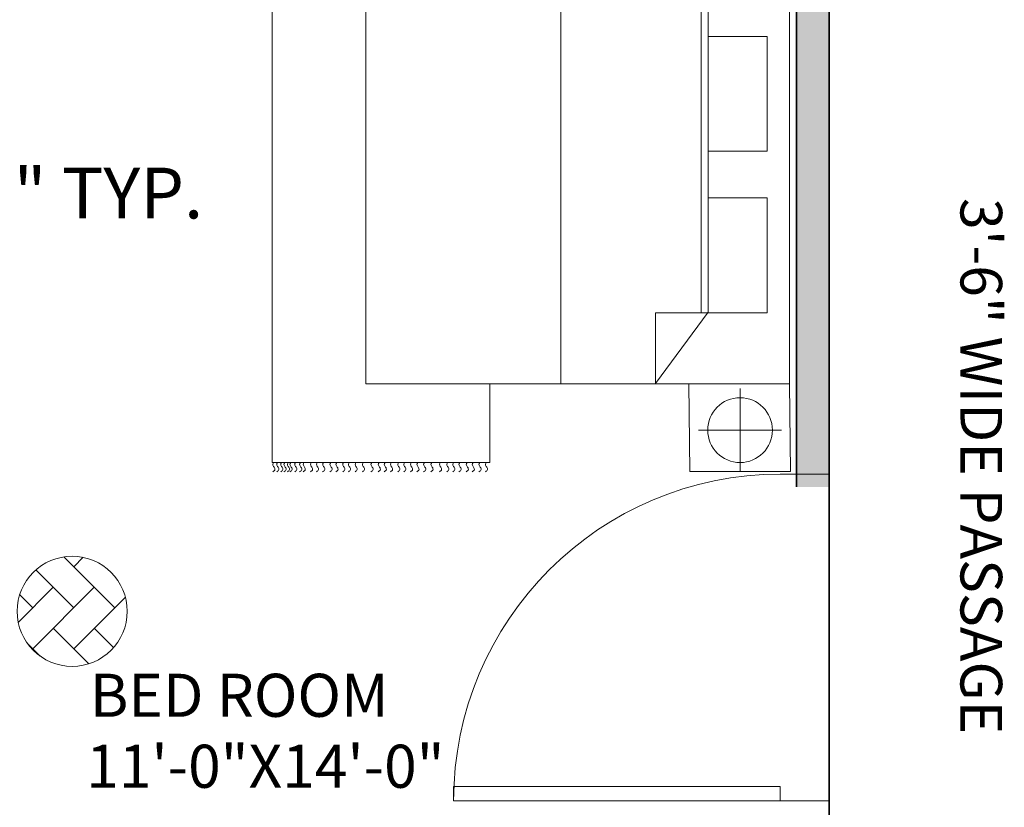
# Model space of a CAD drawing. Units: inches. Extents: x 0 to 4258, y 0 to 3769.
# Tile 21 of 30: x 3708 to 3844, y 3443 to 3552. Entities that reach past the tile are written whole.
import ezdxf

# ---------------------------------------------------------------- set-up
doc = ezdxf.new("R2010")
doc.units = ezdxf.units.IN
doc.header["$MEASUREMENT"] = 0
doc.layers.get('0').update_dxf_attribs({"color": 16})
for name, color, linetype, lineweight in [('A-ANNO-DIMS', 250, 'Continuous', 18), ('A-AREA-IDEN', 250, 'Continuous', 18), ('A-WALL-PATT', 16, 'Continuous', 13), ('doors', 250, 'Continuous', 18), ('furniture', 13, 'Continuous', 18), ('walls', 251, 'Continuous', 35)]:
    doc.layers.add(name, color=color, linetype=linetype, lineweight=lineweight)
doc.styles.get("Standard").update_dxf_attribs({"font": 'arial.ttf'})
doc.dimstyles.get("Standard").update_dxf_attribs({"dimtxt": 7, "dimasz": 0.18, "dimexe": 0.18, "dimexo": 0.0625, "dimgap": 0.09, "dimtad": 0, "dimtih": 1, "dimtoh": 1, "dimzin": 0, "dimdsep": 46, "dimlunit": 3, "dimtxsty": 'Standard', "dimcen": 0.09, "dimadec": 0, "dimazin": 0, "dimtfac": 1, "dimtofl": 0, "dimtmove": 0, "dimatfit": 3, "dimfxl": 1, "dimtolj": 1, "dimtzin": 0, "dimarcsym": 0})

# ---------------------------------------------------------------- blocks, each defined once
blk = doc.blocks.new('CARPET')
at = {"layer": 'furniture'}
for p, q in [((-51.53, -98.11), (-51.53, -55.12)), ((-51.53, -55.12), (-41.27, -55.12)), ((36, -55.12), (51.55, -55.12)), ((51.55, -55.12), (51.55, -98.11)), ((51.55, -98.11), (-51.53, -98.11))]:
    blk.add_line(p, q, dxfattribs=at)
for points, knots in [([(-53.37, -55.99), (-53.22, -55.8), (-52.9, -55.41), (-52.34, -55.8), (-51.89, -56.08), (-51.65, -55.91), (-51.53, -55.83)], [0, 0, 0, 0, 0.653278, 1.290138, 1.740457, 2.114451, 2.114451, 2.114451, 2.114451]), ([(53.37, -55.99), (53.22, -55.8), (52.9, -55.41), (52.34, -55.8), (51.89, -56.08), (51.65, -55.91), (51.53, -55.83)], [0, 0, 0, 0, 0.653278, 1.290138, 1.740457, 2.114451, 2.114451, 2.114451, 2.114451]), ([(-53.37, -57.26), (-53.22, -57.07), (-52.9, -56.67), (-52.34, -57.07), (-51.89, -57.35), (-51.65, -57.17), (-51.53, -57.1)], [0, 0, 0, 0, 0.653278, 1.290138, 1.740457, 2.114451, 2.114451, 2.114451, 2.114451]), ([(-53.37, -58.59), (-53.22, -58.4), (-52.9, -58.01), (-52.34, -58.4), (-51.89, -58.68), (-51.65, -58.5), (-51.53, -58.43)], [0, 0, 0, 0, 0.653278, 1.290138, 1.740457, 2.114451, 2.114451, 2.114451, 2.114451]), ([(53.37, -57.26), (53.22, -57.07), (52.9, -56.67), (52.34, -57.07), (51.89, -57.35), (51.65, -57.17), (51.53, -57.1)], [0, 0, 0, 0, 0.653278, 1.290138, 1.740457, 2.114451, 2.114451, 2.114451, 2.114451]), ([(53.37, -58.59), (53.22, -58.4), (52.9, -58.01), (52.34, -58.4), (51.89, -58.68), (51.65, -58.5), (51.53, -58.43)], [0, 0, 0, 0, 0.653278, 1.290138, 1.740457, 2.114451, 2.114451, 2.114451, 2.114451]), ([(-53.37, -59.78), (-53.22, -59.58), (-52.9, -59.19), (-52.34, -59.58), (-51.89, -59.86), (-51.65, -59.69), (-51.53, -59.61)], [0, 0, 0, 0, 0.653278, 1.290138, 1.740457, 2.114451, 2.114451, 2.114451, 2.114451]), ([(53.37, -59.78), (53.22, -59.58), (52.9, -59.19), (52.34, -59.58), (51.89, -59.86), (51.65, -59.69), (51.53, -59.61)], [0, 0, 0, 0, 0.653278, 1.290138, 1.740457, 2.114451, 2.114451, 2.114451, 2.114451]), ([(-53.37, -61.22), (-53.22, -61.02), (-52.9, -60.63), (-52.34, -61.02), (-51.89, -61.3), (-51.65, -61.13), (-51.53, -61.05)], [0, 0, 0, 0, 0.653278, 1.290138, 1.740457, 2.114451, 2.114451, 2.114451, 2.114451]), ([(-53.37, -62.44), (-53.22, -62.25), (-52.9, -61.86), (-52.34, -62.25), (-51.89, -62.53), (-51.65, -62.36), (-51.53, -62.28)], [0, 0, 0, 0, 0.653278, 1.290138, 1.740457, 2.114451, 2.114451, 2.114451, 2.114451]), ([(53.37, -61.22), (53.22, -61.02), (52.9, -60.63), (52.34, -61.02), (51.89, -61.3), (51.65, -61.13), (51.53, -61.05)], [0, 0, 0, 0, 0.653278, 1.290138, 1.740457, 2.114451, 2.114451, 2.114451, 2.114451]), ([(53.37, -62.44), (53.22, -62.25), (52.9, -61.86), (52.34, -62.25), (51.89, -62.53), (51.65, -62.36), (51.53, -62.28)], [0, 0, 0, 0, 0.653278, 1.290138, 1.740457, 2.114451, 2.114451, 2.114451, 2.114451]), ([(-53.37, -63.63), (-53.22, -63.43), (-52.9, -63.04), (-52.34, -63.43), (-51.89, -63.72), (-51.65, -63.54), (-51.53, -63.46)], [0, 0, 0, 0, 0.653278, 1.290138, 1.740457, 2.114451, 2.114451, 2.114451, 2.114451]), ([(53.37, -63.63), (53.22, -63.43), (52.9, -63.04), (52.34, -63.43), (51.89, -63.72), (51.65, -63.54), (51.53, -63.46)], [0, 0, 0, 0, 0.653278, 1.290138, 1.740457, 2.114451, 2.114451, 2.114451, 2.114451]), ([(-53.37, -65.07), (-53.22, -64.87), (-52.9, -64.48), (-52.34, -64.87), (-51.89, -65.15), (-51.65, -64.98), (-51.53, -64.9)], [0, 0, 0, 0, 0.653278, 1.290138, 1.740457, 2.114451, 2.114451, 2.114451, 2.114451]), ([(53.37, -65.07), (53.22, -64.87), (52.9, -64.48), (52.34, -64.87), (51.89, -65.15), (51.65, -64.98), (51.53, -64.9)], [0, 0, 0, 0, 0.653278, 1.290138, 1.740457, 2.114451, 2.114451, 2.114451, 2.114451]), ([(-53.37, -66.76), (-53.22, -66.56), (-52.9, -66.17), (-52.34, -66.56), (-51.89, -66.84), (-51.65, -66.67), (-51.53, -66.59)], [0, 0, 0, 0, 0.653278, 1.290138, 1.740457, 2.114451, 2.114451, 2.114451, 2.114451]), ([(-53.37, -68.2), (-53.22, -68), (-52.9, -67.61), (-52.34, -68), (-51.89, -68.28), (-51.65, -68.11), (-51.53, -68.03)], [0, 0, 0, 0, 0.653278, 1.290138, 1.740457, 2.114451, 2.114451, 2.114451, 2.114451]), ([(53.37, -66.76), (53.22, -66.56), (52.9, -66.17), (52.34, -66.56), (51.89, -66.84), (51.65, -66.67), (51.53, -66.59)], [0, 0, 0, 0, 0.653278, 1.290138, 1.740457, 2.114451, 2.114451, 2.114451, 2.114451]), ([(53.37, -68.2), (53.22, -68), (52.9, -67.61), (52.34, -68), (51.89, -68.28), (51.65, -68.11), (51.53, -68.03)], [0, 0, 0, 0, 0.653278, 1.290138, 1.740457, 2.114451, 2.114451, 2.114451, 2.114451]), ([(-53.37, -69.53), (-53.22, -69.33), (-52.9, -68.94), (-52.34, -69.33), (-51.89, -69.61), (-51.65, -69.44), (-51.53, -69.36)], [0, 0, 0, 0, 0.653278, 1.290138, 1.740457, 2.114451, 2.114451, 2.114451, 2.114451]), ([(53.37, -69.53), (53.22, -69.33), (52.9, -68.94), (52.34, -69.33), (51.89, -69.61), (51.65, -69.44), (51.53, -69.36)], [0, 0, 0, 0, 0.653278, 1.290138, 1.740457, 2.114451, 2.114451, 2.114451, 2.114451]), ([(-53.37, -70.79), (-53.22, -70.6), (-52.9, -70.21), (-52.34, -70.6), (-51.89, -70.88), (-51.65, -70.7), (-51.53, -70.63)], [0, 0, 0, 0, 0.653278, 1.290138, 1.740457, 2.114451, 2.114451, 2.114451, 2.114451]), ([(-53.37, -72.12), (-53.22, -71.93), (-52.9, -71.54), (-52.34, -71.93), (-51.89, -72.21), (-51.65, -72.04), (-51.53, -71.96)], [0, 0, 0, 0, 0.653278, 1.290138, 1.740457, 2.114451, 2.114451, 2.114451, 2.114451]), ([(53.37, -70.79), (53.22, -70.6), (52.9, -70.21), (52.34, -70.6), (51.89, -70.88), (51.65, -70.7), (51.53, -70.63)], [0, 0, 0, 0, 0.653278, 1.290138, 1.740457, 2.114451, 2.114451, 2.114451, 2.114451]), ([(53.37, -72.12), (53.22, -71.93), (52.9, -71.54), (52.34, -71.93), (51.89, -72.21), (51.65, -72.04), (51.53, -71.96)], [0, 0, 0, 0, 0.653278, 1.290138, 1.740457, 2.114451, 2.114451, 2.114451, 2.114451]), ([(-53.37, -73.31), (-53.22, -73.11), (-52.9, -72.72), (-52.34, -73.11), (-51.89, -73.4), (-51.65, -73.22), (-51.53, -73.14)], [0, 0, 0, 0, 0.653278, 1.290138, 1.740457, 2.114451, 2.114451, 2.114451, 2.114451]), ([(53.37, -73.31), (53.22, -73.11), (52.9, -72.72), (52.34, -73.11), (51.89, -73.4), (51.65, -73.22), (51.53, -73.14)], [0, 0, 0, 0, 0.653278, 1.290138, 1.740457, 2.114451, 2.114451, 2.114451, 2.114451]), ([(-53.37, -74.75), (-53.22, -74.55), (-52.9, -74.16), (-52.34, -74.55), (-51.89, -74.83), (-51.65, -74.66), (-51.53, -74.58)], [0, 0, 0, 0, 0.653278, 1.290138, 1.740457, 2.114451, 2.114451, 2.114451, 2.114451]), ([(-53.37, -75.98), (-53.22, -75.78), (-52.9, -75.39), (-52.34, -75.78), (-51.89, -76.06), (-51.65, -75.89), (-51.53, -75.81)], [0, 0, 0, 0, 0.653278, 1.290138, 1.740457, 2.114451, 2.114451, 2.114451, 2.114451]), ([(53.37, -74.75), (53.22, -74.55), (52.9, -74.16), (52.34, -74.55), (51.89, -74.83), (51.65, -74.66), (51.53, -74.58)], [0, 0, 0, 0, 0.653278, 1.290138, 1.740457, 2.114451, 2.114451, 2.114451, 2.114451]), ([(53.37, -75.98), (53.22, -75.78), (52.9, -75.39), (52.34, -75.78), (51.89, -76.06), (51.65, -75.89), (51.53, -75.81)], [0, 0, 0, 0, 0.653278, 1.290138, 1.740457, 2.114451, 2.114451, 2.114451, 2.114451]), ([(-53.37, -77.16), (-53.22, -76.96), (-52.9, -76.57), (-52.34, -76.96), (-51.89, -77.25), (-51.65, -77.07), (-51.53, -76.99)], [0, 0, 0, 0, 0.653278, 1.290138, 1.740457, 2.114451, 2.114451, 2.114451, 2.114451]), ([(53.37, -77.16), (53.22, -76.96), (52.9, -76.57), (52.34, -76.96), (51.89, -77.25), (51.65, -77.07), (51.53, -76.99)], [0, 0, 0, 0, 0.653278, 1.290138, 1.740457, 2.114451, 2.114451, 2.114451, 2.114451]), ([(-53.37, -78.6), (-53.22, -78.4), (-52.9, -78.01), (-52.34, -78.4), (-51.89, -78.68), (-51.65, -78.51), (-51.53, -78.43)], [0, 0, 0, 0, 0.653278, 1.290138, 1.740457, 2.114451, 2.114451, 2.114451, 2.114451]), ([(53.37, -78.6), (53.22, -78.4), (52.9, -78.01), (52.34, -78.4), (51.89, -78.68), (51.65, -78.51), (51.53, -78.43)], [0, 0, 0, 0, 0.653278, 1.290138, 1.740457, 2.114451, 2.114451, 2.114451, 2.114451]), ([(-53.37, -80.29), (-53.22, -80.09), (-52.9, -79.7), (-52.34, -80.09), (-51.89, -80.37), (-51.65, -80.2), (-51.53, -80.12)], [0, 0, 0, 0, 0.653278, 1.290138, 1.740457, 2.114451, 2.114451, 2.114451, 2.114451]), ([(-53.37, -81.73), (-53.22, -81.53), (-52.9, -81.14), (-52.34, -81.53), (-51.89, -81.81), (-51.65, -81.64), (-51.53, -81.56)], [0, 0, 0, 0, 0.653278, 1.290138, 1.740457, 2.114451, 2.114451, 2.114451, 2.114451]), ([(53.37, -80.29), (53.22, -80.09), (52.9, -79.7), (52.34, -80.09), (51.89, -80.37), (51.65, -80.2), (51.53, -80.12)], [0, 0, 0, 0, 0.653278, 1.290138, 1.740457, 2.114451, 2.114451, 2.114451, 2.114451]), ([(53.37, -81.73), (53.22, -81.53), (52.9, -81.14), (52.34, -81.53), (51.89, -81.81), (51.65, -81.64), (51.53, -81.56)], [0, 0, 0, 0, 0.653278, 1.290138, 1.740457, 2.114451, 2.114451, 2.114451, 2.114451]), ([(-53.37, -83.06), (-53.22, -82.86), (-52.9, -82.47), (-52.34, -82.86), (-51.89, -83.14), (-51.65, -82.97), (-51.53, -82.89)], [0, 0, 0, 0, 0.653278, 1.290138, 1.740457, 2.114451, 2.114451, 2.114451, 2.114451]), ([(53.37, -83.06), (53.22, -82.86), (52.9, -82.47), (52.34, -82.86), (51.89, -83.14), (51.65, -82.97), (51.53, -82.89)], [0, 0, 0, 0, 0.653278, 1.290138, 1.740457, 2.114451, 2.114451, 2.114451, 2.114451]), ([(-53.37, -84.18), (-53.22, -83.99), (-52.9, -83.6), (-52.34, -83.99), (-51.89, -84.27), (-51.65, -84.09), (-51.53, -84.02)], [0, 0, 0, 0, 0.653278, 1.290138, 1.740457, 2.114451, 2.114451, 2.114451, 2.114451]), ([(-53.37, -85.51), (-53.22, -85.32), (-52.9, -84.93), (-52.34, -85.32), (-51.89, -85.6), (-51.65, -85.42), (-51.53, -85.35)], [0, 0, 0, 0, 0.653278, 1.290138, 1.740457, 2.114451, 2.114451, 2.114451, 2.114451]), ([(53.37, -84.18), (53.22, -83.99), (52.9, -83.6), (52.34, -83.99), (51.89, -84.27), (51.65, -84.09), (51.53, -84.02)], [0, 0, 0, 0, 0.653278, 1.290138, 1.740457, 2.114451, 2.114451, 2.114451, 2.114451]), ([(53.37, -85.51), (53.22, -85.32), (52.9, -84.93), (52.34, -85.32), (51.89, -85.6), (51.65, -85.42), (51.53, -85.35)], [0, 0, 0, 0, 0.653278, 1.290138, 1.740457, 2.114451, 2.114451, 2.114451, 2.114451]), ([(-53.37, -86.7), (-53.22, -86.5), (-52.9, -86.11), (-52.34, -86.5), (-51.89, -86.78), (-51.65, -86.61), (-51.53, -86.53)], [0, 0, 0, 0, 0.653278, 1.290138, 1.740457, 2.114451, 2.114451, 2.114451, 2.114451]), ([(53.37, -86.7), (53.22, -86.5), (52.9, -86.11), (52.34, -86.5), (51.89, -86.78), (51.65, -86.61), (51.53, -86.53)], [0, 0, 0, 0, 0.653278, 1.290138, 1.740457, 2.114451, 2.114451, 2.114451, 2.114451]), ([(-53.37, -88.14), (-53.22, -87.94), (-52.9, -87.55), (-52.34, -87.94), (-51.89, -88.22), (-51.65, -88.05), (-51.53, -87.97)], [0, 0, 0, 0, 0.653278, 1.290138, 1.740457, 2.114451, 2.114451, 2.114451, 2.114451]), ([(-53.37, -89.36), (-53.22, -89.17), (-52.9, -88.78), (-52.34, -89.17), (-51.89, -89.45), (-51.65, -89.28), (-51.53, -89.2)], [0, 0, 0, 0, 0.653278, 1.290138, 1.740457, 2.114451, 2.114451, 2.114451, 2.114451]), ([(53.37, -88.14), (53.22, -87.94), (52.9, -87.55), (52.34, -87.94), (51.89, -88.22), (51.65, -88.05), (51.53, -87.97)], [0, 0, 0, 0, 0.653278, 1.290138, 1.740457, 2.114451, 2.114451, 2.114451, 2.114451]), ([(53.37, -89.36), (53.22, -89.17), (52.9, -88.78), (52.34, -89.17), (51.89, -89.45), (51.65, -89.28), (51.53, -89.2)], [0, 0, 0, 0, 0.653278, 1.290138, 1.740457, 2.114451, 2.114451, 2.114451, 2.114451]), ([(-53.37, -90.55), (-53.22, -90.35), (-52.9, -89.96), (-52.34, -90.35), (-51.89, -90.64), (-51.65, -90.46), (-51.53, -90.38)], [0, 0, 0, 0, 0.653278, 1.290138, 1.740457, 2.114451, 2.114451, 2.114451, 2.114451]), ([(53.37, -90.55), (53.22, -90.35), (52.9, -89.96), (52.34, -90.35), (51.9, -90.63), (51.66, -90.47), (51.55, -90.4)], [0, 0, 0, 0, 0.653278, 1.290138, 1.740457, 2.0926, 2.0926, 2.0926, 2.0926]), ([(-53.37, -91.99), (-53.22, -91.79), (-52.9, -91.4), (-52.34, -91.79), (-51.89, -92.07), (-51.65, -91.9), (-51.53, -91.82)], [0, 0, 0, 0, 0.653278, 1.290138, 1.740457, 2.114451, 2.114451, 2.114451, 2.114451]), ([(-53.37, -92.69), (-53.22, -92.48), (-52.9, -92.08), (-52.35, -92.49), (-51.89, -92.77), (-51.65, -92.6), (-51.53, -92.52)], [0, 0, 0, 0, 0.663904, 1.307406, 1.757725, 2.131719, 2.131719, 2.131719, 2.131719]), ([(-53.37, -93.61), (-53.22, -93.42), (-52.9, -93.03), (-52.34, -93.42), (-51.89, -93.7), (-51.65, -93.52), (-51.53, -93.45)], [0, 0, 0, 0, 0.653278, 1.290138, 1.740457, 2.114451, 2.114451, 2.114451, 2.114451]), ([(53.37, -91.99), (53.22, -91.79), (52.9, -91.4), (52.34, -91.79), (51.9, -92.07), (51.66, -91.91), (51.55, -91.83)], [0, 0, 0, 0, 0.653278, 1.290138, 1.740457, 2.0926, 2.0926, 2.0926, 2.0926]), ([(53.37, -92.69), (53.22, -92.49), (52.9, -92.09), (52.34, -92.49), (51.9, -92.77), (51.66, -92.61), (51.55, -92.53)], [0, 0, 0, 0, 0.656792, 1.295826, 1.746145, 2.098292, 2.098292, 2.098292, 2.098292]), ([(53.37, -93.66), (53.22, -93.46), (52.9, -93.07), (52.34, -93.46), (51.9, -93.74), (51.66, -93.58), (51.55, -93.5)], [0, 0, 0, 0, 0.653278, 1.290138, 1.740457, 2.0926, 2.0926, 2.0926, 2.0926]), ([(-53.37, -94.55), (-53.22, -94.35), (-52.9, -93.96), (-52.34, -94.35), (-51.89, -94.63), (-51.65, -94.46), (-51.53, -94.38)], [0, 0, 0, 0, 0.653278, 1.290138, 1.740457, 2.114451, 2.114451, 2.114451, 2.114451]), ([(-53.37, -95.05), (-53.22, -94.85), (-52.9, -94.46), (-52.34, -94.85), (-51.89, -95.14), (-51.65, -94.96), (-51.53, -94.88)], [0, 0, 0, 0, 0.653278, 1.290138, 1.740457, 2.114451, 2.114451, 2.114451, 2.114451]), ([(-53.37, -95.73), (-53.22, -95.54), (-52.9, -95.15), (-52.34, -95.54), (-51.89, -95.82), (-51.65, -95.65), (-51.53, -95.57)], [0, 0, 0, 0, 0.653278, 1.290138, 1.740457, 2.114451, 2.114451, 2.114451, 2.114451]), ([(53.37, -94.59), (53.22, -94.4), (52.9, -94.01), (52.34, -94.4), (51.9, -94.68), (51.66, -94.51), (51.55, -94.44)], [0, 0, 0, 0, 0.653278, 1.290138, 1.740457, 2.0926, 2.0926, 2.0926, 2.0926]), ([(53.37, -95.1), (53.22, -94.9), (52.9, -94.51), (52.34, -94.9), (51.9, -95.18), (51.66, -95.02), (51.55, -94.94)], [0, 0, 0, 0, 0.653278, 1.290138, 1.740457, 2.0926, 2.0926, 2.0926, 2.0926]), ([(-53.37, -96.38), (-53.22, -96.18), (-52.9, -95.79), (-52.34, -96.18), (-51.89, -96.47), (-51.65, -96.29), (-51.53, -96.21)], [0, 0, 0, 0, 0.653278, 1.290138, 1.740457, 2.114451, 2.114451, 2.114451, 2.114451]), ([(-53.37, -97.17), (-53.22, -96.98), (-52.9, -96.59), (-52.34, -96.98), (-51.89, -97.26), (-51.65, -97.08), (-51.53, -97.01)], [0, 0, 0, 0, 0.653278, 1.290138, 1.740457, 2.114451, 2.114451, 2.114451, 2.114451]), ([(53.37, -95.78), (53.22, -95.58), (52.9, -95.19), (52.34, -95.58), (51.89, -95.86), (51.65, -95.69), (51.53, -95.61)], [0, 0, 0, 0, 0.653278, 1.290138, 1.740457, 2.114451, 2.114451, 2.114451, 2.114451]), ([(53.37, -96.43), (53.22, -96.23), (52.9, -95.84), (52.34, -96.23), (51.89, -96.51), (51.65, -96.34), (51.53, -96.26)], [0, 0, 0, 0, 0.653278, 1.290138, 1.740457, 2.114451, 2.114451, 2.114451, 2.114451]), ([(53.37, -97.22), (53.22, -97.02), (52.9, -96.63), (52.34, -97.02), (51.89, -97.3), (51.65, -97.13), (51.53, -97.05)], [0, 0, 0, 0, 0.653278, 1.290138, 1.740457, 2.114451, 2.114451, 2.114451, 2.114451]), ([(-53.37, -97.99), (-53.22, -97.79), (-52.9, -97.4), (-52.34, -97.79), (-51.89, -98.08), (-51.65, -97.9), (-51.53, -97.82)], [0, 0, 0, 0, 0.653278, 1.290138, 1.740457, 2.114451, 2.114451, 2.114451, 2.114451]), ([(53.37, -97.99), (53.22, -97.79), (52.9, -97.4), (52.34, -97.79), (51.89, -98.08), (51.65, -97.9), (51.53, -97.82)], [0, 0, 0, 0, 0.653278, 1.290138, 1.740457, 2.114451, 2.114451, 2.114451, 2.114451])]:
    blk.add_open_spline(points, degree=3, knots=knots, dxfattribs=at)
blk = doc.blocks.new('A$C58D270C6')
at = {"layer": 'furniture'}
for p, q in [((9.09, 124.13), (9.09, 108.87)), ((1.46, 116.5), (16.73, 116.5)), ((14.97, 94.84), (24.62, 107.92)), ((24.62, 94.93), (24.62, 107.92)), ((42.08, 108), (42.08, 36)), ((14.97, 94.93), (24.62, 94.93)), ((14.97, 94.84), (14.97, 36)), ((16.22, 94.93), (16.22, 36)), ((9.25, 36), (9.25, 20.74)), ((1.62, 28.37), (16.88, 28.37))]:
    blk.add_line(p, q, dxfattribs=at)
for points in [[(18.5, 108), (18.34, 124.13), (-0.16, 124.13), (0, 108)], [(0, 108), (77.91, 108), (77.91, 36), (0, 36)], [(4.09, 94.93), (14.97, 94.93), (14.97, 73.83), (4.09, 73.83)], [(4.09, 65.23), (14.97, 65.23), (14.97, 44.13), (4.09, 44.13)], [(18.65, 19.87), (18.5, 36), (0, 36), (0.16, 19.87)]]:
    blk.add_lwpolyline(points, close=True, dxfattribs=at)
for centre in [(9.09, 116.5), (9.25, 28.37)]:
    blk.add_circle(centre, 5.95, dxfattribs=at)
at = {"layer": 'furniture', "xscale": 0.9312884925094044, "yscale": 0.9312884925094044, "zscale": 0.9312884925094044, "rotation": 90}
blk.add_blockref('CARPET', (3.79, 74.47), dxfattribs=at)
blk = doc.blocks.new('*U23')
for p, q in [((0, 0), (0, -6)), ((40, 0), (40, -6))]:
    blk.add_line(p, q)
blk.add_lwpolyline([(0, 0), (0, 40), (1.75, 40), (1.75, 0)], close=True)
blk.add_arc((0, 0), 40, 0, 90)
blk = doc.blocks.new('SEATING-TWO-CHAIRS-AND-TABLE')
h = blk.add_hatch()
h.set_pattern_fill('AR-HBONE', color=256, angle=90)
h.set_pattern_definition([(135, (3403.542, -4056.0025), (-5.6568542, 3e-16), [12, -4]), (225, (3400.7137, -4053.174), (-5.6568542, 8e-16), [12, -4])])
h.paths.add_polyline_path([(7.59, 14.04, 1), (7.59, 29.23, 1)])
for p, q in [((30.53, 40.83), (30.5, 44.11)), ((19.25, 25.7), (19.25, 40.83)), ((23.18, 41.34), (30.53, 41.34)), ((23.18, 25.19), (30.53, 25.19)), ((30.63, 22.02), (30.63, 25.19)), ((30.53, 18.81), (30.5, 22.09)), ((23.18, 19.32), (30.53, 19.32)), ((19.25, 3.68), (19.25, 18.81)), ((23.18, 3.17), (30.53, 3.17)), ((30.63, 0), (30.63, 3.17))]:
    blk.add_line(p, q)
blk.add_circle((7.59, 21.64), 7.59)
for centre, radius, start, end in [((23.25, 33.02), 13.25, 303.8239, 56.829), ((21.94, 35.53), 5.94, 77.9198, 116.8624), ((22.13, 33.01), 11.48, 317.0375, 42.9625), ((21.94, 31), 5.94, 243.1376, 282.0802), ((23.25, 11.01), 13.25, 303.8239, 56.829), ((21.94, 13.51), 5.94, 77.9198, 116.8624), ((22.13, 10.99), 11.48, 317.0375, 42.9625), ((21.94, 8.98), 5.94, 243.1376, 282.0802)]:
    blk.add_arc(centre, radius, start, end)
blk = doc.blocks.new('*D36')
at = {"layer": 'A-ANNO-DIMS', "color": 0, "lineweight": -2, "transparency": 16777216}
for p, q in [((3690.88, 3548.93), (3697.37, 3548.93)), ((3697.19, 3548.75), (3697.19, 3531.4)), ((3697.19, 3506.63), (3697.19, 3523.98)), ((3690.88, 3506.45), (3697.37, 3506.45))]:
    blk.add_line(p, q, dxfattribs=at)
at = {"layer": 'A-ANNO-DIMS', "color": 0, "transparency": 16777216}
for points in [[(3697.16, 3548.75), (3697.22, 3548.75), (3697.19, 3548.93)], [(3697.16, 3506.63), (3697.22, 3506.63), (3697.19, 3506.45)]]:
    blk.add_solid(points, dxfattribs=at)
at = {"layer": 'Defpoints', "color": 0, "transparency": 16777216}
for p in [(3690.82, 3548.93), (3697.19, 3548.93), (3690.82, 3506.45)]:
    blk.add_point(p, dxfattribs=at)
at = {"layer": 'A-ANNO-DIMS', "color": 0, "transparency": 16777216, "insert": (3697.19, 3527.69), "char_height": 7, "attachment_point": 5}
blk.add_mtext('\\A1;TV 3\'-6 1/2" TYP.', dxfattribs=at)

msp = doc.modelspace()

# ---------------------------------------------------------------- hatches: boundary and pattern name
at = {"layer": 'A-WALL-PATT'}
h = msp.add_hatch(color=256, dxfattribs=at)
h.dxf.hatch_style = 1
h.paths.add_polyline_path([(3819.804, 3598.293), (3815.304, 3598.293), (3815.304, 3487.182), (3819.804, 3487.182)])

# ---------------------------------------------------------------- linework, layer by layer
at = {"layer": 'walls'}
for p, q in [((3815.304, 3487.182), (3815.304, 3598.293)), ((3819.804, 3421.293), (3819.804, 3598.293))]:
    msp.add_line(p, q, dxfattribs=at)

# ---------------------------------------------------------------- block references
at = {"layer": 'doors', "xscale": 1.125993190768673, "yscale": 1.125993190768673, "zscale": 1.125993190768673, "rotation": 90.00000000000003}
msp.add_blockref('*U23', (3813.048, 3443.897), dxfattribs=at)
at = {"layer": 'furniture', "xscale": 0.7500000390647866, "yscale": 0.7500000390647866, "zscale": 0.7500000390647866, "rotation": 180}
msp.add_blockref('A$C58D270C6', (3814.348, 3582.385), dxfattribs=at)
at = {"layer": 'furniture', "rotation": 180}
msp.add_blockref('SEATING-TWO-CHAIRS-AND-TABLE', (3722.972, 3491.674), dxfattribs=at)

# ---------------------------------------------------------------- texts
at = {"layer": 'A-AREA-IDEN'}
msp.add_text('3\'-6" WIDE PASSAGE', height=5.74671, rotation=270, dxfattribs=at).set_placement((3837.938, 3526.987))
for s, height, p in [('BED ROOM', 5.939, (3717.823, 3455.49)), ('11\'-0"X14\'-0"', 5.93898, (3717.326, 3445.708))]:
    msp.add_text(s, height=height, dxfattribs=at).set_placement(p)

# ---------------------------------------------------------------- dimensions: what is measured, and where the dimension line sits
at = {"layer": 'A-ANNO-DIMS'}
dim = msp.add_linear_dim(base=(3697.187, 3548.926), p1=(3690.816, 3506.452), p2=(3690.816, 3548.926), angle=90, text='TV <> TYP.', dimstyle='Standard', override={"dimdec": 1, "dimlfac": 1, "dimrnd": 0, "dimzin": 1, "dimdsep": 46, "dimlunit": 4, "dimfrac": 2}, dxfattribs=at)
dim.commit()
dim.dimension.update_dxf_attribs({"geometry": '*D36', "text_midpoint": (3697.187, 3527.689)})

doc.saveas('drawing.dxf')
